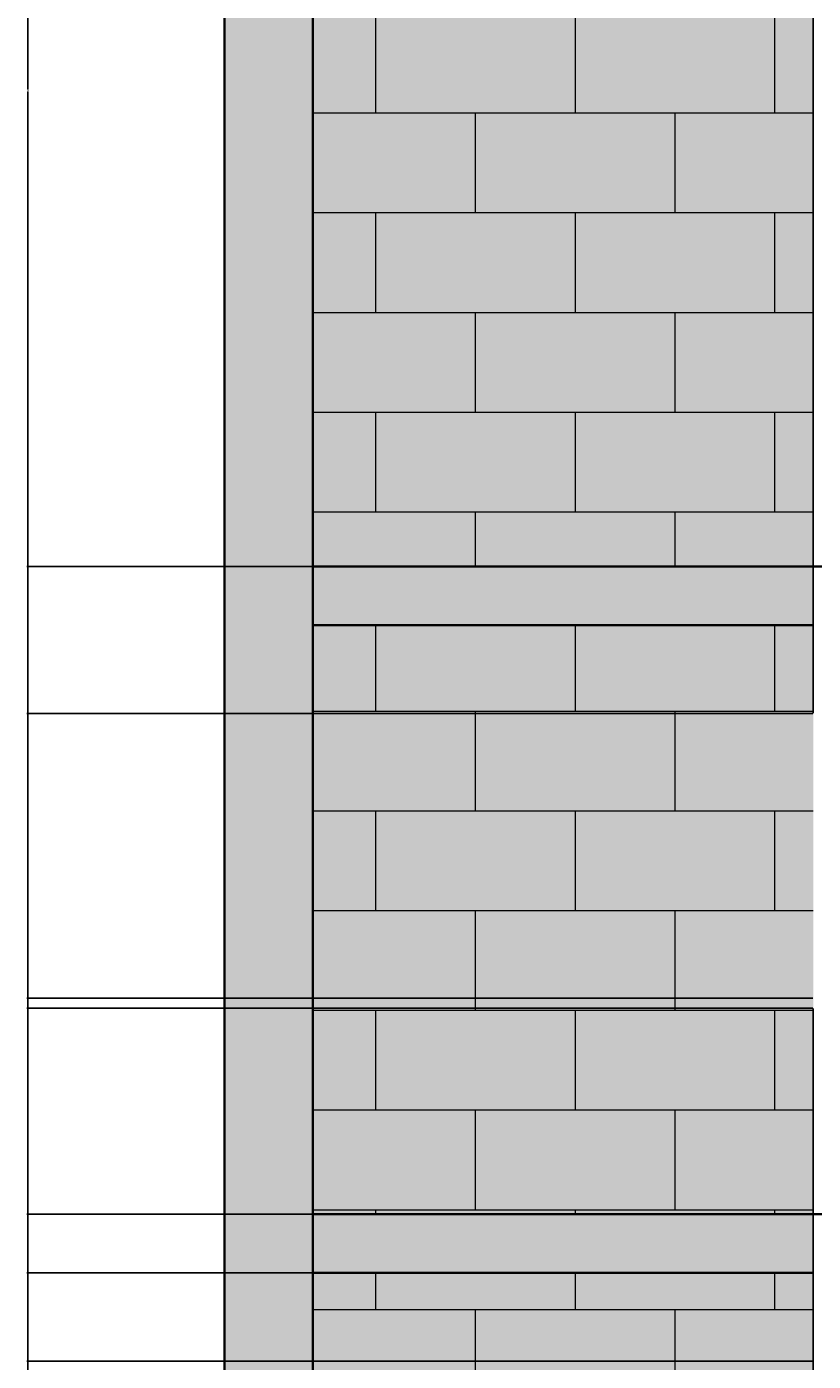
# Model space of a CAD drawing. Units: inches. Extents: x 2794 to 3619, y 522 to 1397.
# Tile 2 of 10: x 2794 to 2954, y 701 to 973. Entities that reach past the tile are written whole.
import ezdxf

# ---------------------------------------------------------------- set-up
doc = ezdxf.new("R2010")
doc.units = ezdxf.units.IN
for name, color, linetype, lineweight in [('A-ANNO-DIMS', 2, 'Continuous', 18), ('A-ELEV', 7, 'Continuous', 35), ('A-ELEV-PATT', 8, 'Continuous', 13)]:
    doc.layers.add(name, color=color, linetype=linetype, lineweight=lineweight)
doc.styles.get("Standard").update_dxf_attribs({"font": 'arial.ttf'})
doc.dimstyles.get("Standard").update_dxf_attribs({"dimtxt": 0.18, "dimasz": 0.18, "dimexe": 0.18, "dimexo": 0.0625, "dimgap": 0.09, "dimtad": 0, "dimtih": 1, "dimtoh": 1, "dimdec": 4, "dimzin": 0, "dimdsep": 46, "dimtxsty": 'Standard', "dimcen": 0.09, "dimadec": 0, "dimazin": 0, "dimtfac": 1, "dimtdec": 4, "dimtofl": 0, "dimtmove": 0, "dimatfit": 3, "dimfxl": 1, "dimtolj": 1, "dimtzin": 0, "dimarcsym": 0})

# ---------------------------------------------------------------- blocks, each defined once
blk = doc.blocks.new('*D16')
at = {"layer": 'A-ANNO-DIMS', "color": 0, "lineweight": -2, "transparency": 16777216}
for p, q in [((3142.2, 1356.64), (2793.99, 1356.64)), ((2794.17, 1356.46), (2794.17, 959.82)), ((2794.17, 562.82), (2794.17, 959.45)), ((2834.2, 562.64), (2793.99, 562.64))]:
    blk.add_line(p, q, dxfattribs=at)
at = {"layer": 'A-ANNO-DIMS', "color": 0, "transparency": 16777216}
for points in [[(2794.14, 1356.46), (2794.2, 1356.46), (2794.17, 1356.64)], [(2794.14, 562.82), (2794.2, 562.82), (2794.17, 562.64)]]:
    blk.add_solid(points, dxfattribs=at)
at = {"layer": 'Defpoints', "color": 0, "transparency": 16777216}
for p in [(2794.17, 1356.64), (3142.27, 1356.64), (2834.27, 562.64)]:
    blk.add_point(p, dxfattribs=at)
at = {"layer": 'A-ANNO-DIMS', "color": 0, "transparency": 16777216, "insert": (2794.17, 959.64), "char_height": 0.18, "attachment_point": 5}
blk.add_mtext('\\A1;794', dxfattribs=at)
blk = doc.blocks.new('*D25')
at = {"layer": 'A-ANNO-DIMS', "color": 0, "lineweight": -2, "transparency": 16777216}
for p, q in [((2852.2, 730.64), (2793.99, 730.64)), ((2794.17, 730.46), (2794.17, 724.82)), ((2794.17, 718.82), (2794.17, 724.45)), ((2852.2, 718.64), (2793.99, 718.64))]:
    blk.add_line(p, q, dxfattribs=at)
at = {"layer": 'A-ANNO-DIMS', "color": 0, "transparency": 16777216}
for points in [[(2794.14, 730.46), (2794.2, 730.46), (2794.17, 730.64)], [(2794.14, 718.82), (2794.2, 718.82), (2794.17, 718.64)]]:
    blk.add_solid(points, dxfattribs=at)
at = {"layer": 'Defpoints', "color": 0, "transparency": 16777216}
for p in [(2794.17, 730.64), (2852.27, 730.64), (2852.27, 718.64)]:
    blk.add_point(p, dxfattribs=at)
at = {"layer": 'A-ANNO-DIMS', "color": 0, "transparency": 16777216, "insert": (2794.17, 724.64), "char_height": 0.18, "attachment_point": 5}
blk.add_mtext('\\A1;12', dxfattribs=at)
blk = doc.blocks.new('*D28')
at = {"layer": 'A-ANNO-DIMS', "color": 0, "lineweight": -2, "transparency": 16777216}
for p, q in [((2954.27, 832.7), (2954.27, 1396.92)), ((2954.45, 1396.74), (2972.05, 1396.74)), ((2990.09, 1396.74), (2972.48, 1396.74)), ((2990.27, 820.7), (2990.27, 1396.92))]:
    blk.add_line(p, q, dxfattribs=at)
at = {"layer": 'A-ANNO-DIMS', "color": 0, "transparency": 16777216}
for points in [[(2954.45, 1396.77), (2954.45, 1396.71), (2954.27, 1396.74)], [(2990.09, 1396.77), (2990.09, 1396.71), (2990.27, 1396.74)]]:
    blk.add_solid(points, dxfattribs=at)
at = {"layer": 'Defpoints', "color": 0, "transparency": 16777216}
for p in [(2990.27, 1396.74), (2954.27, 832.64), (2990.27, 820.64)]:
    blk.add_point(p, dxfattribs=at)
at = {"layer": 'A-ANNO-DIMS', "color": 0, "transparency": 16777216, "insert": (2972.27, 1396.74), "char_height": 0.18, "attachment_point": 5}
blk.add_mtext('\\A1;36', dxfattribs=at)
blk = doc.blocks.new('*D32')
at = {"layer": 'A-ANNO-DIMS', "color": 0, "lineweight": -2, "transparency": 16777216}
for p, q in [((2954.27, 772.57), (2954.27, 522.36)), ((2958.83, 730.57), (2958.83, 522.36)), ((2954.45, 522.54), (2956.17, 522.54)), ((2958.65, 522.54), (2956.93, 522.54))]:
    blk.add_line(p, q, dxfattribs=at)
at = {"layer": 'A-ANNO-DIMS', "color": 0, "transparency": 16777216}
for points in [[(2954.45, 522.57), (2954.45, 522.51), (2954.27, 522.54)], [(2958.65, 522.57), (2958.65, 522.51), (2958.83, 522.54)]]:
    blk.add_solid(points, dxfattribs=at)
at = {"layer": 'Defpoints', "color": 0, "transparency": 16777216}
for p in [(2954.27, 772.64), (2958.83, 730.64), (2958.83, 522.54)]:
    blk.add_point(p, dxfattribs=at)
at = {"layer": 'A-ANNO-DIMS', "color": 0, "transparency": 16777216, "insert": (2956.55, 522.54), "char_height": 0.18, "attachment_point": 5}
blk.add_mtext('\\A1;4.561', dxfattribs=at)
blk = doc.blocks.new('*D38')
at = {"layer": 'A-ANNO-DIMS', "color": 0, "lineweight": -2, "transparency": 16777216}
for p, q in [((2958.76, 730.64), (2793.99, 730.64)), ((2794.17, 730.46), (2794.17, 715.82)), ((2794.17, 700.82), (2794.17, 715.45)), ((2954.2, 700.64), (2793.99, 700.64))]:
    blk.add_line(p, q, dxfattribs=at)
at = {"layer": 'A-ANNO-DIMS', "color": 0, "transparency": 16777216}
for points in [[(2794.14, 730.46), (2794.2, 730.46), (2794.17, 730.64)], [(2794.14, 700.82), (2794.2, 700.82), (2794.17, 700.64)]]:
    blk.add_solid(points, dxfattribs=at)
at = {"layer": 'Defpoints', "color": 0, "transparency": 16777216}
for p in [(2794.17, 730.64), (2958.83, 730.64), (2954.27, 700.64)]:
    blk.add_point(p, dxfattribs=at)
at = {"layer": 'A-ANNO-DIMS', "color": 0, "transparency": 16777216, "insert": (2794.17, 715.64), "char_height": 0.18, "attachment_point": 5}
blk.add_mtext('\\A1;30', dxfattribs=at)
blk = doc.blocks.new('*D39')
at = {"layer": 'A-ANNO-DIMS', "color": 0, "lineweight": -2, "transparency": 16777216}
for p, q in [((2954.2, 772.64), (2793.99, 772.64)), ((2794.17, 772.46), (2794.17, 751.82)), ((2794.17, 730.82), (2794.17, 751.45)), ((2958.76, 730.64), (2793.99, 730.64))]:
    blk.add_line(p, q, dxfattribs=at)
at = {"layer": 'A-ANNO-DIMS', "color": 0, "transparency": 16777216}
for points in [[(2794.14, 772.46), (2794.2, 772.46), (2794.17, 772.64)], [(2794.14, 730.82), (2794.2, 730.82), (2794.17, 730.64)]]:
    blk.add_solid(points, dxfattribs=at)
at = {"layer": 'Defpoints', "color": 0, "transparency": 16777216}
for p in [(2794.17, 772.64), (2954.27, 772.64), (2958.83, 730.64)]:
    blk.add_point(p, dxfattribs=at)
at = {"layer": 'A-ANNO-DIMS', "color": 0, "transparency": 16777216, "insert": (2794.17, 751.64), "char_height": 0.18, "attachment_point": 5}
blk.add_mtext('\\A1;42', dxfattribs=at)
blk = doc.blocks.new('*D40')
at = {"layer": 'A-ANNO-DIMS', "color": 0, "lineweight": -2, "transparency": 16777216}
for p, q in [((2954.2, 774.64), (2793.99, 774.64)), ((2954.2, 772.64), (2793.99, 772.64)), ((2794.17, 774.46), (2794.17, 773.82)), ((2794.17, 772.82), (2794.17, 773.45))]:
    blk.add_line(p, q, dxfattribs=at)
at = {"layer": 'A-ANNO-DIMS', "color": 0, "transparency": 16777216}
for points in [[(2794.14, 774.46), (2794.2, 774.46), (2794.17, 774.64)], [(2794.14, 772.82), (2794.2, 772.82), (2794.17, 772.64)]]:
    blk.add_solid(points, dxfattribs=at)
at = {"layer": 'Defpoints', "color": 0, "transparency": 16777216}
for p in [(2794.17, 774.64), (2954.27, 774.64), (2954.27, 772.64)]:
    blk.add_point(p, dxfattribs=at)
at = {"layer": 'A-ANNO-DIMS', "color": 0, "transparency": 16777216, "insert": (2794.17, 773.64), "char_height": 0.18, "attachment_point": 5}
blk.add_mtext('\\A1;2', dxfattribs=at)
blk = doc.blocks.new('*D41')
at = {"layer": 'A-ANNO-DIMS', "color": 0, "lineweight": -2, "transparency": 16777216}
for p, q in [((2954.2, 832.64), (2793.99, 832.64)), ((2794.17, 832.46), (2794.17, 803.82)), ((2794.17, 774.82), (2794.17, 803.45)), ((2954.2, 774.64), (2793.99, 774.64))]:
    blk.add_line(p, q, dxfattribs=at)
at = {"layer": 'A-ANNO-DIMS', "color": 0, "transparency": 16777216}
for points in [[(2794.14, 832.46), (2794.2, 832.46), (2794.17, 832.64)], [(2794.14, 774.82), (2794.2, 774.82), (2794.17, 774.64)]]:
    blk.add_solid(points, dxfattribs=at)
at = {"layer": 'Defpoints', "color": 0, "transparency": 16777216}
for p in [(2794.17, 832.64), (2954.27, 832.64), (2954.27, 774.64)]:
    blk.add_point(p, dxfattribs=at)
at = {"layer": 'A-ANNO-DIMS', "color": 0, "transparency": 16777216, "insert": (2794.17, 803.64), "char_height": 0.18, "attachment_point": 5}
blk.add_mtext('\\A1;58', dxfattribs=at)
blk = doc.blocks.new('*D42')
at = {"layer": 'A-ANNO-DIMS', "color": 0, "lineweight": -2, "transparency": 16777216}
for p, q in [((2958.76, 862.64), (2793.99, 862.64)), ((2794.17, 862.46), (2794.17, 847.82)), ((2794.17, 832.82), (2794.17, 847.45)), ((2954.2, 832.64), (2793.99, 832.64))]:
    blk.add_line(p, q, dxfattribs=at)
at = {"layer": 'A-ANNO-DIMS', "color": 0, "transparency": 16777216}
for points in [[(2794.14, 862.46), (2794.2, 862.46), (2794.17, 862.64)], [(2794.14, 832.82), (2794.2, 832.82), (2794.17, 832.64)]]:
    blk.add_solid(points, dxfattribs=at)
at = {"layer": 'Defpoints', "color": 0, "transparency": 16777216}
for p in [(2794.17, 862.64), (2958.83, 862.64), (2954.27, 832.64)]:
    blk.add_point(p, dxfattribs=at)
at = {"layer": 'A-ANNO-DIMS', "color": 0, "transparency": 16777216, "insert": (2794.17, 847.64), "char_height": 0.18, "attachment_point": 5}
blk.add_mtext('\\A1;30', dxfattribs=at)

msp = doc.modelspace()

# ---------------------------------------------------------------- hatches: boundary and pattern name
at = {"layer": 'A-ELEV-PATT', "transparency": 33554687}
h = msp.add_hatch(color=256, dxfattribs=at)
h.dxf.hatch_style = 1
h.paths.add_polyline_path([(3578.2659, 1294.6351), (3560.2659, 1294.6351), (3560.2659, 642.6351), (3578.2659, 642.6351)])
h.paths.add_polyline_path([(2852.2659, 1294.6351), (2834.2659, 1294.6351), (2834.2659, 642.6351), (2852.2659, 642.6351)])
h = msp.add_hatch(color=256, dxfattribs=at)
h.dxf.hatch_style = 1
h.paths.add_polyline_path([(2852.2659, 1294.6351), (2834.2659, 1294.6351), (2834.2659, 562.6351), (2852.2659, 562.6351)])
h.paths.add_polyline_path([(3578.2659, 1294.6351), (3560.2659, 1294.6351), (3560.2659, 562.6351), (3578.2659, 562.6351)])
h = msp.add_hatch(color=256, dxfattribs=at)
h.dxf.hatch_style = 1
h.paths.add_polyline_path([(2852.2659, 1246.6351), (2954.2659, 1246.6351), (2954.2659, 1258.6351), (2900.2659, 1258.6351), (2900.2659, 1294.6351), (2852.2659, 1294.6351)])
h.paths.add_polyline_path([(3512.2659, 1294.6351), (3512.2659, 1258.6351), (3458.2659, 1258.6351), (3458.2659, 1246.6351), (3560.2659, 1246.6351), (3560.2659, 1294.6351)])
h.paths.add_polyline_path([(2954.2659, 1114.6351), (2954.2659, 1126.6351), (2852.2659, 1126.6351), (2852.2659, 1114.6351)])
h.paths.add_polyline_path([(3560.2659, 1114.6351), (3560.2659, 1126.6351), (3458.2659, 1126.6351), (3458.2659, 1114.6351)])
h.paths.add_polyline_path([(3560.2659, 982.6351), (3560.2659, 994.6351), (3458.2659, 994.6351), (3458.2659, 982.6351)])
h.paths.add_polyline_path([(2954.2659, 982.6351), (2954.2659, 994.6351), (2852.2659, 994.6351), (2852.2659, 982.6351)])
h.paths.add_polyline_path([(2852.2659, 862.6351), (2852.2659, 850.6351), (2954.2659, 850.6351), (2954.2659, 862.6351)])
h.paths.add_polyline_path([(2852.2659, 730.6351), (2852.2659, 718.6351), (2954.2659, 718.6351), (2954.2659, 730.6351)])
h.paths.add_polyline_path([(3560.2659, 718.6351), (3560.2659, 730.6351), (3458.2659, 730.6351), (3458.2659, 718.6351)])
h.paths.add_polyline_path([(3560.2659, 850.6351), (3560.2659, 862.6351), (3458.2659, 862.6351), (3458.2659, 850.6351)])
at = {"layer": 'A-ELEV-PATT'}
h = msp.add_hatch(dxfattribs=at)
h.set_pattern_fill('AR-B816', color=256, scale=0.1)
h.paths.add_polyline_path([(2954.2659, 1114.6351), (2852.2659, 1114.6351), (2852.2659, 994.6351), (2954.2659, 994.6351)])
h.paths.add_polyline_path([(2954.2659, 1246.6351), (2852.2659, 1246.6351), (2852.2659, 1126.6351), (2954.2659, 1126.6351)])
h.paths.add_polyline_path([(2954.2659, 982.6351), (2852.2659, 982.6351), (2852.2659, 862.6351), (2954.2659, 862.6351)])
h.paths.add_polyline_path([(2954.2659, 850.6351), (2852.2659, 850.6351), (2852.2659, 730.6351), (2954.2659, 730.6351)])
h.paths.add_polyline_path([(3560.2659, 850.6351), (3458.2659, 850.6351), (3458.2659, 730.6351), (3560.2659, 730.6351)])
h.paths.add_polyline_path([(3560.2659, 982.6351), (3458.2659, 982.6351), (3458.2659, 862.6351), (3560.2659, 862.6351)])
h.paths.add_polyline_path([(3560.2659, 1114.6351), (3458.2659, 1114.6351), (3458.2659, 994.6351), (3560.2659, 994.6351)])
h.paths.add_polyline_path([(3560.2659, 1246.6351), (3458.2659, 1246.6351), (3458.2659, 1126.6351), (3560.2659, 1126.6351)])
h.paths.add_polyline_path([(2852.2659, 642.6351), (2954.2659, 642.6351), (2954.2659, 718.6351), (2852.2659, 718.6351)])
h.paths.add_polyline_path([(3458.2659, 640.6351), (3560.2659, 640.6351), (3560.2659, 718.6351), (3458.2659, 718.6351)])
at = {"layer": 'A-ELEV-PATT', "transparency": 33554630}
h = msp.add_hatch(color=256, dxfattribs=at)
h.dxf.hatch_style = 1
h.paths.add_polyline_path([(2954.2659, 1114.6351), (2852.2659, 1114.6351), (2852.2659, 994.6351), (2954.2659, 994.6351)])
h.paths.add_polyline_path([(2954.2659, 982.6351), (2852.2659, 982.6351), (2852.2659, 862.6351), (2954.2659, 862.6351)])
h.paths.add_polyline_path([(2954.2659, 850.6351), (2852.2659, 850.6351), (2852.2659, 730.6351), (2954.2659, 730.6351)])
h.paths.add_polyline_path([(3560.2659, 850.6351), (3458.2659, 850.6351), (3458.2659, 730.6351), (3560.2659, 730.6351)])
h.paths.add_polyline_path([(3560.2659, 982.6351), (3458.2659, 982.6351), (3458.2659, 862.6351), (3560.2659, 862.6351)])
h.paths.add_polyline_path([(3560.2659, 1114.6351), (3458.2659, 1114.6351), (3458.2659, 994.6351), (3560.2659, 994.6351)])
h.paths.add_polyline_path([(3560.2659, 1246.6351), (3458.2659, 1246.6351), (3458.2659, 1126.6351), (3560.2659, 1126.6351)])
h.paths.add_polyline_path([(2852.2659, 642.6351), (2954.2659, 642.6351), (2954.2659, 718.6351), (2852.2659, 718.6351)])
h.paths.add_polyline_path([(3458.2659, 642.6351), (3560.2659, 642.6351), (3560.2659, 718.6351), (3458.2659, 718.6351)])

# ---------------------------------------------------------------- linework, layer by layer
at = {"layer": 'A-ELEV'}
for p, q in [((2834.2659, 562.6351), (2834.2659, 1297.6351)), ((2852.2659, 562.6351), (2852.2659, 1294.6351)), ((3146.2659, 862.6351), (2852.2659, 862.6351)), ((2954.2659, 850.6351), (2852.2659, 850.6351)), ((3150.2659, 730.6351), (2852.2659, 730.6351)), ((2954.2659, 718.6351), (2852.2659, 718.6351))]:
    msp.add_line(p, q, dxfattribs=at)

# ---------------------------------------------------------------- dimensions: what is measured, and where the dimension line sits
at = {"layer": 'A-ANNO-DIMS'}
for base, p1, p2, override, picture, middle in [((2990.2659, 1396.7351), (2954.2659, 832.6351), (2990.2659, 820.6351), {"dimdec": 0, "dimlfac": 1, "dimrnd": 0, "dimzin": 0, "dimdsep": 46, "dimlunit": 2}, '*D28', (2972.2659, 1396.7351)), ((2958.8268, 522.5351), (2954.2659, 772.6351), (2958.8268, 730.6351), {"dimdec": 3, "dimlfac": 1, "dimrnd": 0, "dimzin": 0, "dimdsep": 46, "dimlunit": 2}, '*D32', (2956.5463, 522.5351))]:
    dim = msp.add_linear_dim(base=base, p1=p1, p2=p2, dimstyle='Standard', override=override, dxfattribs=at)
    dim.commit()
    dim.dimension.update_dxf_attribs({"geometry": picture, "text_midpoint": middle})
for base, p1, p2, picture, middle in [((2794.1659, 1356.6351), (2834.2659, 562.6351), (3142.2659, 1356.6351), '*D16', (2794.1659, 959.6351)), ((2794.1659, 862.6351), (2954.2659, 832.6351), (2958.8268, 862.6351), '*D42', (2794.1659, 847.6351)), ((2794.1659, 832.6351), (2954.2659, 774.6351), (2954.2659, 832.6351), '*D41', (2794.1659, 803.6351)), ((2794.1659, 774.6351), (2954.2659, 772.6351), (2954.2659, 774.6351), '*D40', (2794.1659, 773.6351)), ((2794.1659, 772.6351), (2958.8268, 730.6351), (2954.2659, 772.6351), '*D39', (2794.1659, 751.6351)), ((2794.1659, 730.6351), (2852.2659, 718.6351), (2852.2659, 730.6351), '*D25', (2794.1659, 724.6351)), ((2794.1659, 730.6351), (2954.2659, 700.6351), (2958.8268, 730.6351), '*D38', (2794.1659, 715.6351))]:
    dim = msp.add_linear_dim(base=base, p1=p1, p2=p2, angle=90, dimstyle='Standard', override={"dimdec": 0, "dimlfac": 1, "dimrnd": 0, "dimzin": 0, "dimdsep": 46, "dimlunit": 2}, dxfattribs=at)
    dim.commit()
    dim.dimension.update_dxf_attribs({"geometry": picture, "text_midpoint": middle})

doc.saveas('drawing.dxf')
